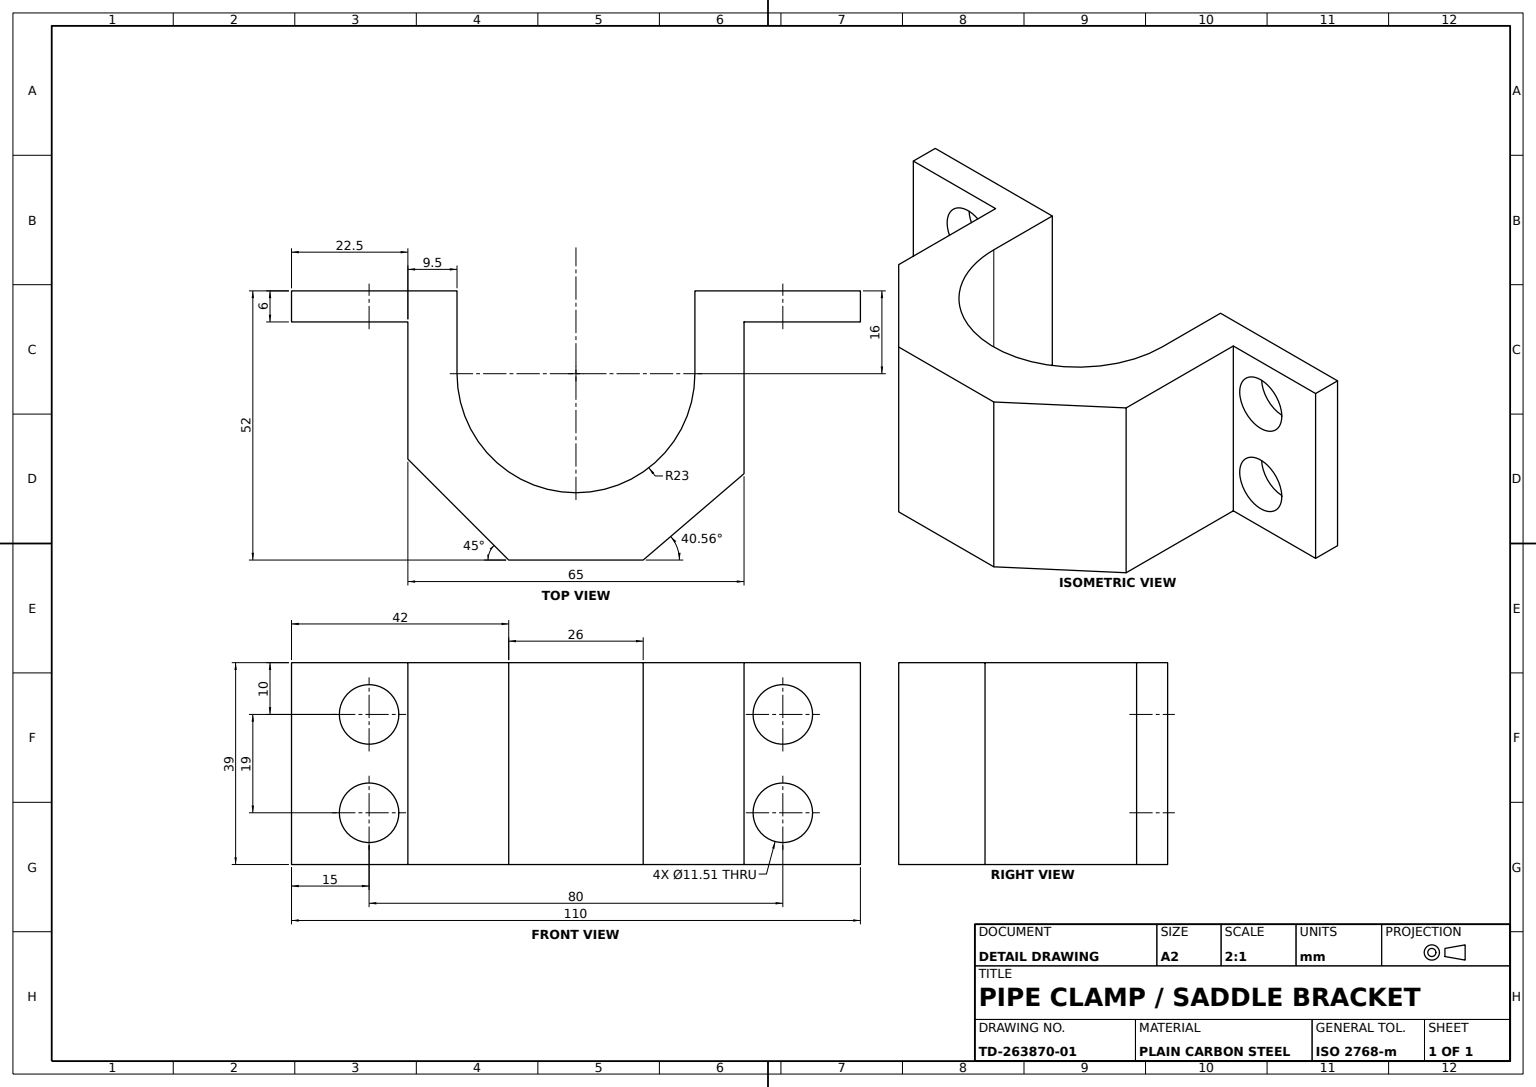
from build123d import *

# Parameters (mm, degrees)
SADDLE_BODY_DEPTH       = 19.5
FLANGE_HOLES_SKETCH_R   = 5.754759715
FLANGE_BOLT_HOLES_DEPTH = 39


with BuildPart() as part:
    # Saddle Profile Sketch → Saddle Body (new, symmetric)
    with BuildSketch(Plane(origin=(0, 0, 0), x_dir=(1, 0, 0), z_dir=(0, 1, 0))):
        with BuildLine():
            Line((-23, -0.309929889), (-23, -16.309929889))
            ThreePointArc((-23, -16.309929889), (0, -39.309929889), (23, -16.309929889))
            Line((23, -16.309929889), (23, -0.309929889))
            Line((23, -0.309929889), (55, -0.309929889))
            Line((55, -0.309929889), (55, -6.309929889))
            Line((55, -6.309929889), (32.5, -6.309929889))
            Line((32.5, -6.309929889), (32.5, -35.619251923))
            Line((32.5, -35.619251923), (13, -52.309929889))
            Line((13, -52.309929889), (-13, -52.309929889))
            Line((-13, -52.309929889), (-32.5, -32.809929889))
            Line((-32.5, -32.809929889), (-32.5, -6.309929889))
            Line((-32.5, -6.309929889), (-55, -6.309929889))
            Line((-55, -6.309929889), (-55, -0.309929889))
            Line((-55, -0.309929889), (-23, -0.309929889))
        make_face()
    extrude(amount=SADDLE_BODY_DEPTH, both=True)

    # Flange Holes Sketch → Flange Bolt Holes (cut)
    with BuildSketch(Plane(origin=(0, 0, 0.309929889), x_dir=(-1, 0, 0), z_dir=(0, 0, -1))):
        with Locations((-40, 9.5)):
            Circle(FLANGE_HOLES_SKETCH_R)
        with Locations((40, 9.5)):
            Circle(FLANGE_HOLES_SKETCH_R)
        with Locations((40, -9.5)):
            Circle(FLANGE_HOLES_SKETCH_R)
        with Locations((-40, -9.5)):
            Circle(FLANGE_HOLES_SKETCH_R)
    extrude(amount=-FLANGE_BOLT_HOLES_DEPTH, mode=Mode.SUBTRACT)


solid = part.part
